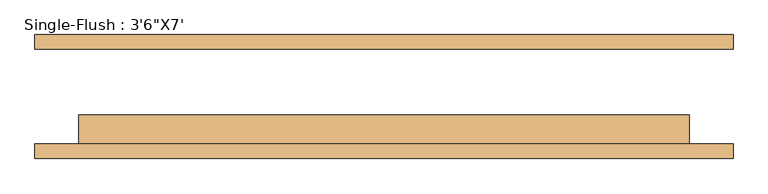
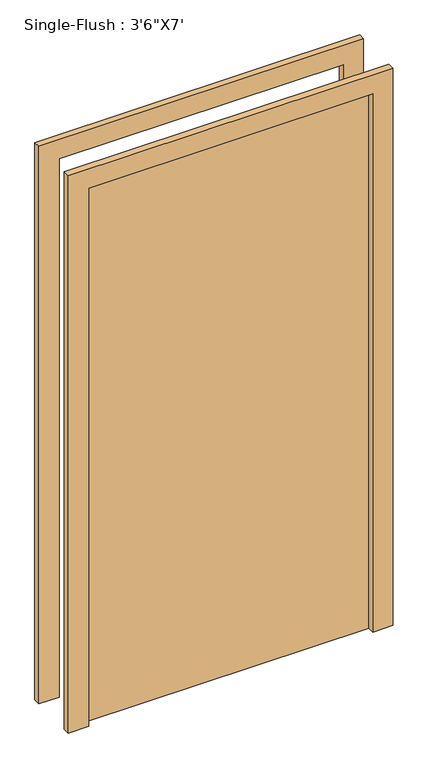
"""IFC4 building model written with IfcOpenShell, lengths in millimetres: door geometry."""

from ifc_helpers import new_model, si_unit, frame, origin, origin_with_axes, place, context, project, spatial, polyline, outline, extrude, source, transform, mapped, element, save


def door_bd8f54db(model_context):
    return source(origin(), model_context, "Body", "SweptSolid", [
        extrude(outline(polyline([(2209.8, -609.6), (0.0, -609.6), (0.0, -533.4), (2133.6, -533.4), (2133.6, 533.4), (0.0, 533.4), (0.0, 609.6), (2209.8, 609.6), (2209.8, -609.6)])), frame((0.0, -108.3, 0.0), z_axis=(0.0, 1.0, 0.0), x_axis=(0.0, 0.0, 1.0)), (0.0, 0.0, 1.0), 25.4),
        extrude(outline(polyline([(2209.8, 609.6), (2209.8, -609.6), (0.0, -609.6), (0.0, -533.4), (2133.6, -533.4), (2133.6, 533.4), (0.0, 533.4), (0.0, 609.6), (2209.8, 609.6)])), frame((0.0, 82.9, 0.0), z_axis=(0.0, 1.0, 0.0), x_axis=(0.0, 0.0, 1.0)), (0.0, 0.0, 1.0), 25.4),
        extrude(outline(polyline([(533.4, -32.1), (533.4, -82.9), (-533.4, -82.9), (-533.4, -32.1), (533.4, -32.1)])), origin_with_axes(), (0.0, 0.0, 1.0), 2133.6),
    ])


if __name__ == "__main__":
    model = new_model("IFC4")
    model_context = context("Model", 3, world=origin())
    ifc_project = project(units=[si_unit("LENGTHUNIT", "METRE", prefix="MILLI")], contexts=[model_context])
    site = spatial("IfcSite", under=ifc_project)
    building = spatial("IfcBuilding", under=site)
    placement = place(None, origin())
    door_shape = door_bd8f54db(model_context)
    element("IfcDoor", 1, ObjectType="Single-Flush : 3'6\"X7'", at=placement, inside=building, context=model_context, shape_type="MappedRepresentation", body=[
        mapped(door_shape, transform((0.0, 0.0, 0.0), x_axis=(1.0, 0.0, 0.0), y_axis=(0.0, 1.0, 0.0), z_axis=(0.0, 0.0, 1.0))),
    ])
    save(model, "model.ifc")

# Revit data of these elements
# Type "Single-Flush : 3'6\"X7'"
#   Type Mark = "8"
#   Assembly Code = "C1020"
#   Thickness = 0' - 2"
#   Height = 7' - 0"
#   Trim Projection Ext = 0' - 1"
#   Trim Projection Int = 0' - 1"
#   Trim Width = 0' - 3"
#   Width = 3' - 6"
#   Door Material = Door - Panel
#   Frame Material = Door - Frame
#   Function = (empty or 0)
#   Wall Closure = (empty or 0)
# Element 1 (IfcDoor, "Single-Flush : 3'6\"X7'")
#   Materials on its faces: "Door - Frame", "Door - Panel"
# Materials
#   "Door - Panel": class "Wood", colour RGB 114 82 51, transparency 0
#   "Door - Frame": colour RGB 153 76 43, transparency 0
